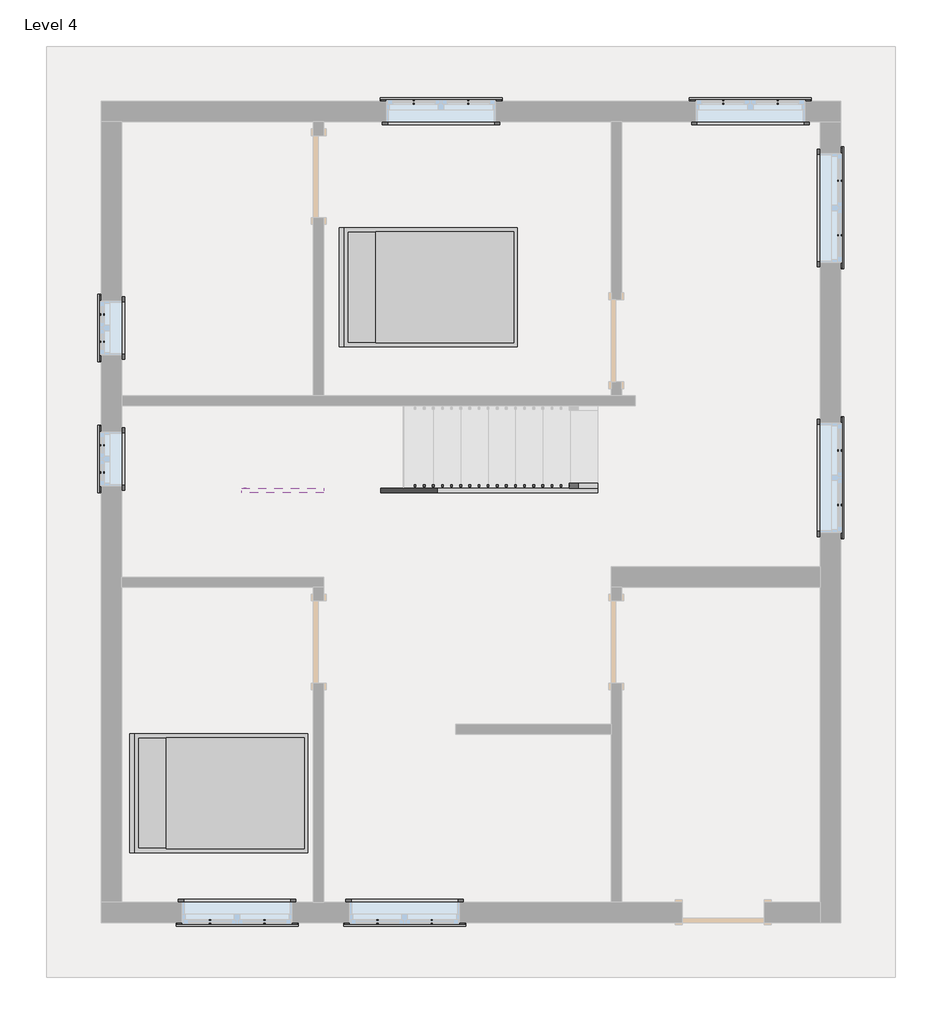
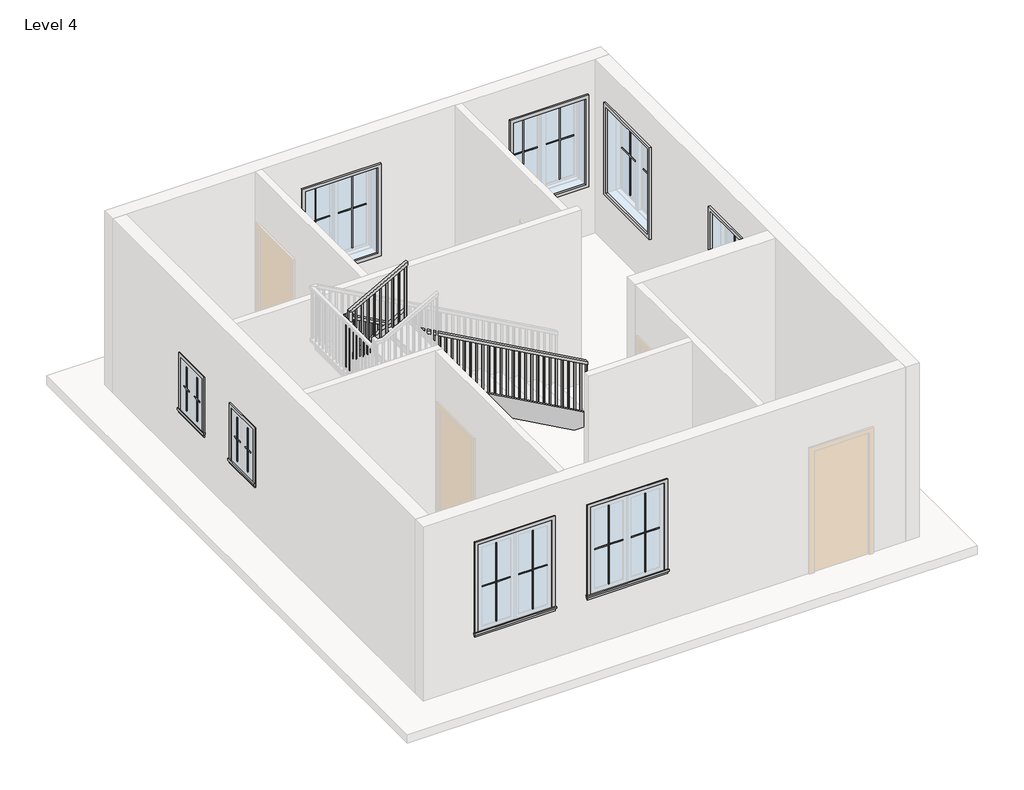
# One storey, part 2 of 2: 32 proxies, 3 members, 2 furniture elements, 1 railing.
"""IFC4 building model written with IfcOpenShell, lengths in millimetres."""

from ifc_helpers import new_model, si_unit, frame, origin, place, context, project, spatial, polyline, outline, extrude, faceted_brep, transform, mapped, element, save
from components import muntin_pattern_2x2_muntin_pattern_2x2_53152e2c, muntin_pattern_2x2_muntin_pattern_2x2_e8f3e573, muntin_pattern_2x2_muntin_pattern_2x2_6dad3731, muntin_pattern_2x2_muntin_pattern_2x2_a30a3345, trim_window_exterior_flat_with_sill_a665a915, trim_window_exterior_flat_with_sill_92b9b949, trim_window_interior_flat_picture_frame_d485c387, trim_window_interior_flat_picture_frame_3bb882cf, bed_17739_bed_17739_15c61121

model = new_model("IFC4")

# Units and contexts
model_context = context("Model", 3, world=origin())
ifc_project = project(units=[si_unit("LENGTHUNIT", "METRE", prefix="MILLI")], contexts=[model_context])

# Site, building, storey
site = spatial("IfcSite", under=ifc_project)
building = spatial("IfcBuilding", under=site)
storey = spatial("IfcBuildingStorey", under=building, Name="Level 4", Elevation=9144.0)

# Proxies
placement = place(None, origin())
muntin_pattern_2x2_muntin_pattern_2x2_shape = muntin_pattern_2x2_muntin_pattern_2x2_53152e2c(model_context)
element("IfcBuildingElementProxy", 1, Name="Muntin Pattern_2x2 : Muntin Pattern_2x2", ObjectType="Muntin Pattern_2x2 : Muntin Pattern_2x2", at=placement, inside=storey, context=model_context, shape_type="MappedRepresentation", body=[
    mapped(muntin_pattern_2x2_muntin_pattern_2x2_shape, transform((1279.525, 12101.9997886, 10128.25), x_axis=(0.0, 1.0, 0.0), y_axis=(-1.0, 0.0, 0.0), z_axis=(0.0, 0.0, 1.0))),
])
element("IfcBuildingElementProxy", 2, Name="Muntin Pattern_2x2 : Muntin Pattern_2x2", ObjectType="Muntin Pattern_2x2 : Muntin Pattern_2x2", at=placement, inside=storey, context=model_context, shape_type="MappedRepresentation", body=[
    mapped(muntin_pattern_2x2_muntin_pattern_2x2_shape, transform((1279.525, 10644.6747886, 10128.25), x_axis=(0.0, 1.0, 0.0), y_axis=(-1.0, 0.0, 0.0), z_axis=(0.0, 0.0, 1.0))),
])
muntin_pattern_2x2_muntin_pattern_2x2_2_shape = muntin_pattern_2x2_muntin_pattern_2x2_e8f3e573(model_context)
element("IfcBuildingElementProxy", 3, Name="Muntin Pattern_2x2 : Muntin Pattern_2x2", ObjectType="Muntin Pattern_2x2 : Muntin Pattern_2x2", at=placement, inside=storey, context=model_context, shape_type="MappedRepresentation", body=[
    mapped(muntin_pattern_2x2_muntin_pattern_2x2_2_shape, transform((1279.525, 12403.6247886, 10128.25), x_axis=(0.0, -1.0, 0.0), y_axis=(1.0, 0.0, 0.0), z_axis=(0.0, 0.0, 1.0))),
])
element("IfcBuildingElementProxy", 4, Name="Muntin Pattern_2x2 : Muntin Pattern_2x2", ObjectType="Muntin Pattern_2x2 : Muntin Pattern_2x2", at=placement, inside=storey, context=model_context, shape_type="MappedRepresentation", body=[
    mapped(muntin_pattern_2x2_muntin_pattern_2x2_2_shape, transform((1279.525, 10946.2997886, 10128.25), x_axis=(0.0, -1.0, 0.0), y_axis=(1.0, 0.0, 0.0), z_axis=(0.0, 0.0, 1.0))),
])
muntin_pattern_2x2_muntin_pattern_2x2_3_shape = muntin_pattern_2x2_muntin_pattern_2x2_6dad3731(model_context)
element("IfcBuildingElementProxy", 5, Name="Muntin Pattern_2x2 : Muntin Pattern_2x2", ObjectType="Muntin Pattern_2x2 : Muntin Pattern_2x2", at=placement, inside=storey, context=model_context, shape_type="MappedRepresentation", body=[
    mapped(muntin_pattern_2x2_muntin_pattern_2x2_3_shape, transform((9490.075, 13892.6997886, 10128.25), x_axis=(0.0, -1.0, 0.0), y_axis=(1.0, 0.0, 0.0), z_axis=(0.0, 0.0, 1.0))),
])
element("IfcBuildingElementProxy", 6, Name="Muntin Pattern_2x2 : Muntin Pattern_2x2", ObjectType="Muntin Pattern_2x2 : Muntin Pattern_2x2", at=placement, inside=storey, context=model_context, shape_type="MappedRepresentation", body=[
    mapped(muntin_pattern_2x2_muntin_pattern_2x2_3_shape, transform((8193.0875, 14767.4122886, 10128.25), x_axis=(1.0, 0.0, 0.0), y_axis=(0.0, 1.0, 0.0), z_axis=(0.0, 0.0, 1.0))),
])
element("IfcBuildingElementProxy", 7, Name="Muntin Pattern_2x2 : Muntin Pattern_2x2", ObjectType="Muntin Pattern_2x2 : Muntin Pattern_2x2", at=placement, inside=storey, context=model_context, shape_type="MappedRepresentation", body=[
    mapped(muntin_pattern_2x2_muntin_pattern_2x2_3_shape, transform((4749.8, 14767.4122886, 10128.25), x_axis=(1.0, 0.0, 0.0), y_axis=(0.0, 1.0, 0.0), z_axis=(0.0, 0.0, 1.0))),
])
element("IfcBuildingElementProxy", 8, Name="Muntin Pattern_2x2 : Muntin Pattern_2x2", ObjectType="Muntin Pattern_2x2 : Muntin Pattern_2x2", at=placement, inside=storey, context=model_context, shape_type="MappedRepresentation", body=[
    mapped(muntin_pattern_2x2_muntin_pattern_2x2_3_shape, transform((9490.075, 10889.1497886, 10128.25), x_axis=(0.0, -1.0, 0.0), y_axis=(1.0, 0.0, 0.0), z_axis=(0.0, 0.0, 1.0))),
])
element("IfcBuildingElementProxy", 9, Name="Muntin Pattern_2x2 : Muntin Pattern_2x2", ObjectType="Muntin Pattern_2x2 : Muntin Pattern_2x2", at=placement, inside=storey, context=model_context, shape_type="MappedRepresentation", body=[
    mapped(muntin_pattern_2x2_muntin_pattern_2x2_3_shape, transform((4950.6207347, 5642.4622886, 10128.25), x_axis=(-1.0, 0.0, 0.0), y_axis=(0.0, -1.0, 0.0), z_axis=(0.0, 0.0, 1.0))),
])
element("IfcBuildingElementProxy", 10, Name="Muntin Pattern_2x2 : Muntin Pattern_2x2", ObjectType="Muntin Pattern_2x2 : Muntin Pattern_2x2", at=placement, inside=storey, context=model_context, shape_type="MappedRepresentation", body=[
    mapped(muntin_pattern_2x2_muntin_pattern_2x2_3_shape, transform((3086.1019847, 5642.4622886, 10128.25), x_axis=(-1.0, 0.0, 0.0), y_axis=(0.0, -1.0, 0.0), z_axis=(0.0, 0.0, 1.0))),
])
muntin_pattern_2x2_muntin_pattern_2x2_4_shape = muntin_pattern_2x2_muntin_pattern_2x2_a30a3345(model_context)
element("IfcBuildingElementProxy", 11, Name="Muntin Pattern_2x2 : Muntin Pattern_2x2", ObjectType="Muntin Pattern_2x2 : Muntin Pattern_2x2", at=placement, inside=storey, context=model_context, shape_type="MappedRepresentation", body=[
    mapped(muntin_pattern_2x2_muntin_pattern_2x2_4_shape, transform((9490.075, 13286.2747886, 10128.25), x_axis=(0.0, 1.0, 0.0), y_axis=(-1.0, 0.0, 0.0), z_axis=(0.0, 0.0, 1.0))),
])
element("IfcBuildingElementProxy", 12, Name="Muntin Pattern_2x2 : Muntin Pattern_2x2", ObjectType="Muntin Pattern_2x2 : Muntin Pattern_2x2", at=placement, inside=storey, context=model_context, shape_type="MappedRepresentation", body=[
    mapped(muntin_pattern_2x2_muntin_pattern_2x2_4_shape, transform((8799.5125, 14767.4122886, 10128.25), x_axis=(-1.0, 0.0, 0.0), y_axis=(0.0, -1.0, 0.0), z_axis=(0.0, 0.0, 1.0))),
])
element("IfcBuildingElementProxy", 13, Name="Muntin Pattern_2x2 : Muntin Pattern_2x2", ObjectType="Muntin Pattern_2x2 : Muntin Pattern_2x2", at=placement, inside=storey, context=model_context, shape_type="MappedRepresentation", body=[
    mapped(muntin_pattern_2x2_muntin_pattern_2x2_4_shape, transform((5356.225, 14767.4122886, 10128.25), x_axis=(-1.0, 0.0, 0.0), y_axis=(0.0, -1.0, 0.0), z_axis=(0.0, 0.0, 1.0))),
])
element("IfcBuildingElementProxy", 14, Name="Muntin Pattern_2x2 : Muntin Pattern_2x2", ObjectType="Muntin Pattern_2x2 : Muntin Pattern_2x2", at=placement, inside=storey, context=model_context, shape_type="MappedRepresentation", body=[
    mapped(muntin_pattern_2x2_muntin_pattern_2x2_4_shape, transform((9490.075, 10282.7247886, 10128.25), x_axis=(0.0, 1.0, 0.0), y_axis=(-1.0, 0.0, 0.0), z_axis=(0.0, 0.0, 1.0))),
])
element("IfcBuildingElementProxy", 15, Name="Muntin Pattern_2x2 : Muntin Pattern_2x2", ObjectType="Muntin Pattern_2x2 : Muntin Pattern_2x2", at=placement, inside=storey, context=model_context, shape_type="MappedRepresentation", body=[
    mapped(muntin_pattern_2x2_muntin_pattern_2x2_4_shape, transform((4344.1957347, 5642.4622886, 10128.25), x_axis=(1.0, 0.0, 0.0), y_axis=(0.0, 1.0, 0.0), z_axis=(0.0, 0.0, 1.0))),
])
element("IfcBuildingElementProxy", 16, Name="Muntin Pattern_2x2 : Muntin Pattern_2x2", ObjectType="Muntin Pattern_2x2 : Muntin Pattern_2x2", at=placement, inside=storey, context=model_context, shape_type="MappedRepresentation", body=[
    mapped(muntin_pattern_2x2_muntin_pattern_2x2_4_shape, transform((2479.6769847, 5642.4622886, 10128.25), x_axis=(1.0, 0.0, 0.0), y_axis=(0.0, 1.0, 0.0), z_axis=(0.0, 0.0, 1.0))),
])
trim_window_exterior_flat_with_sill_shape = trim_window_exterior_flat_with_sill_a665a915(model_context)
element("IfcBuildingElementProxy", 17, Name="Trim-Window-Exterior-Flat : with Sill", ObjectType="Trim-Window-Exterior-Flat : with Sill", at=placement, inside=storey, context=model_context, shape_type="MappedRepresentation", body=[
    mapped(trim_window_exterior_flat_with_sill_shape, transform((1270.0, 12252.8122886, 10972.8), x_axis=(0.0, -1.0, 0.0), y_axis=(0.0, 0.0, 1.0), z_axis=(-1.0, 0.0, 0.0))),
])
element("IfcBuildingElementProxy", 18, Name="Trim-Window-Exterior-Flat : with Sill", ObjectType="Trim-Window-Exterior-Flat : with Sill", at=placement, inside=storey, context=model_context, shape_type="MappedRepresentation", body=[
    mapped(trim_window_exterior_flat_with_sill_shape, transform((1270.0, 10795.4872886, 10972.8), x_axis=(0.0, -1.0, 0.0), y_axis=(0.0, 0.0, 1.0), z_axis=(-1.0, 0.0, 0.0))),
])
trim_window_exterior_flat_with_sill_2_shape = trim_window_exterior_flat_with_sill_92b9b949(model_context)
element("IfcBuildingElementProxy", 19, Name="Trim-Window-Exterior-Flat : with Sill", ObjectType="Trim-Window-Exterior-Flat : with Sill", at=placement, inside=storey, context=model_context, shape_type="MappedRepresentation", body=[
    mapped(trim_window_exterior_flat_with_sill_2_shape, transform((9499.6, 13589.4872886, 11582.4), x_axis=(0.0, 1.0, 0.0), y_axis=(0.0, 0.0, 1.0), z_axis=(1.0, 0.0, 0.0))),
])
element("IfcBuildingElementProxy", 20, Name="Trim-Window-Exterior-Flat : with Sill", ObjectType="Trim-Window-Exterior-Flat : with Sill", at=placement, inside=storey, context=model_context, shape_type="MappedRepresentation", body=[
    mapped(trim_window_exterior_flat_with_sill_2_shape, transform((8496.3, 14776.9372886, 11582.4), x_axis=(-1.0, 0.0, 0.0), y_axis=(0.0, 0.0, 1.0), z_axis=(0.0, 1.0, 0.0))),
])
element("IfcBuildingElementProxy", 21, Name="Trim-Window-Exterior-Flat : with Sill", ObjectType="Trim-Window-Exterior-Flat : with Sill", at=placement, inside=storey, context=model_context, shape_type="MappedRepresentation", body=[
    mapped(trim_window_exterior_flat_with_sill_2_shape, transform((5053.0125, 14776.9372886, 11582.4), x_axis=(-1.0, 0.0, 0.0), y_axis=(0.0, 0.0, 1.0), z_axis=(0.0, 1.0, 0.0))),
])
element("IfcBuildingElementProxy", 22, Name="Trim-Window-Exterior-Flat : with Sill", ObjectType="Trim-Window-Exterior-Flat : with Sill", at=placement, inside=storey, context=model_context, shape_type="MappedRepresentation", body=[
    mapped(trim_window_exterior_flat_with_sill_2_shape, transform((9499.6, 10585.9372886, 11582.4), x_axis=(0.0, 1.0, 0.0), y_axis=(0.0, 0.0, 1.0), z_axis=(1.0, 0.0, 0.0))),
])
element("IfcBuildingElementProxy", 23, Name="Trim-Window-Exterior-Flat : with Sill", ObjectType="Trim-Window-Exterior-Flat : with Sill", at=placement, inside=storey, context=model_context, shape_type="MappedRepresentation", body=[
    mapped(trim_window_exterior_flat_with_sill_2_shape, transform((4647.4082347, 5632.9372886, 11582.4), x_axis=(1.0, 0.0, 0.0), y_axis=(0.0, 0.0, 1.0), z_axis=(0.0, -1.0, 0.0))),
])
element("IfcBuildingElementProxy", 24, Name="Trim-Window-Exterior-Flat : with Sill", ObjectType="Trim-Window-Exterior-Flat : with Sill", at=placement, inside=storey, context=model_context, shape_type="MappedRepresentation", body=[
    mapped(trim_window_exterior_flat_with_sill_2_shape, transform((2782.8894847, 5632.9372886, 11582.4), x_axis=(1.0, 0.0, 0.0), y_axis=(0.0, 0.0, 1.0), z_axis=(0.0, -1.0, 0.0))),
])
trim_window_interior_flat_picture_frame_shape = trim_window_interior_flat_picture_frame_d485c387(model_context)
element("IfcBuildingElementProxy", 25, Name="Trim-Window-Interior-Flat : Picture Frame", ObjectType="Trim-Window-Interior-Flat : Picture Frame", at=placement, inside=storey, context=model_context, shape_type="MappedRepresentation", body=[
    mapped(trim_window_interior_flat_picture_frame_shape, transform((1498.6, 12252.8122886, 10972.8), x_axis=(0.0, 1.0, 0.0), y_axis=(0.0, 0.0, 1.0), z_axis=(1.0, 0.0, 0.0))),
])
element("IfcBuildingElementProxy", 26, Name="Trim-Window-Interior-Flat : Picture Frame", ObjectType="Trim-Window-Interior-Flat : Picture Frame", at=placement, inside=storey, context=model_context, shape_type="MappedRepresentation", body=[
    mapped(trim_window_interior_flat_picture_frame_shape, transform((1498.6, 10795.4872886, 10972.8), x_axis=(0.0, 1.0, 0.0), y_axis=(0.0, 0.0, 1.0), z_axis=(1.0, 0.0, 0.0))),
])
trim_window_interior_flat_picture_frame_2_shape = trim_window_interior_flat_picture_frame_3bb882cf(model_context)
element("IfcBuildingElementProxy", 27, Name="Trim-Window-Interior-Flat : Picture Frame", ObjectType="Trim-Window-Interior-Flat : Picture Frame", at=placement, inside=storey, context=model_context, shape_type="MappedRepresentation", body=[
    mapped(trim_window_interior_flat_picture_frame_2_shape, transform((9271.0, 13589.4872886, 11582.4), x_axis=(0.0, -1.0, 0.0), y_axis=(0.0, 0.0, 1.0), z_axis=(-1.0, 0.0, 0.0))),
])
element("IfcBuildingElementProxy", 28, Name="Trim-Window-Interior-Flat : Picture Frame", ObjectType="Trim-Window-Interior-Flat : Picture Frame", at=placement, inside=storey, context=model_context, shape_type="MappedRepresentation", body=[
    mapped(trim_window_interior_flat_picture_frame_2_shape, transform((8496.3, 14548.3372886, 11582.4), x_axis=(1.0, 0.0, 0.0), y_axis=(0.0, 0.0, 1.0), z_axis=(0.0, -1.0, 0.0))),
])
element("IfcBuildingElementProxy", 29, Name="Trim-Window-Interior-Flat : Picture Frame", ObjectType="Trim-Window-Interior-Flat : Picture Frame", at=placement, inside=storey, context=model_context, shape_type="MappedRepresentation", body=[
    mapped(trim_window_interior_flat_picture_frame_2_shape, transform((5053.0125, 14548.3372886, 11582.4), x_axis=(1.0, 0.0, 0.0), y_axis=(0.0, 0.0, 1.0), z_axis=(0.0, -1.0, 0.0))),
])
element("IfcBuildingElementProxy", 30, Name="Trim-Window-Interior-Flat : Picture Frame", ObjectType="Trim-Window-Interior-Flat : Picture Frame", at=placement, inside=storey, context=model_context, shape_type="MappedRepresentation", body=[
    mapped(trim_window_interior_flat_picture_frame_2_shape, transform((9271.0, 10585.9372886, 11582.4), x_axis=(0.0, -1.0, 0.0), y_axis=(0.0, 0.0, 1.0), z_axis=(-1.0, 0.0, 0.0))),
])
element("IfcBuildingElementProxy", 31, Name="Trim-Window-Interior-Flat : Picture Frame", ObjectType="Trim-Window-Interior-Flat : Picture Frame", at=placement, inside=storey, context=model_context, shape_type="MappedRepresentation", body=[
    mapped(trim_window_interior_flat_picture_frame_2_shape, transform((4647.4082347, 5861.5372886, 11582.4), x_axis=(-1.0, 0.0, 0.0), y_axis=(0.0, 0.0, 1.0), z_axis=(0.0, 1.0, 0.0))),
])
element("IfcBuildingElementProxy", 32, Name="Trim-Window-Interior-Flat : Picture Frame", ObjectType="Trim-Window-Interior-Flat : Picture Frame", at=placement, inside=storey, context=model_context, shape_type="MappedRepresentation", body=[
    mapped(trim_window_interior_flat_picture_frame_2_shape, transform((2782.8894847, 5861.5372886, 11582.4), x_axis=(-1.0, 0.0, 0.0), y_axis=(0.0, 0.0, 1.0), z_axis=(0.0, 1.0, 0.0))),
])

# Furniture
bed_17739_bed_17739_shape = bed_17739_bed_17739_15c61121(model_context)
element("IfcFurniture", 33, ObjectType="Bed_17739 : Bed_17739", at=placement, inside=storey, context=model_context, shape_type="MappedRepresentation", body=[
    mapped(bed_17739_bed_17739_shape, transform((4933.95, 12706.8372886, 9144.0), x_axis=(0.0, 1.0, 0.0), y_axis=(-1.0, 0.0, 0.0), z_axis=(0.0, 0.0, 1.0))),
])
element("IfcFurniture", 34, ObjectType="Bed_17739 : Bed_17739", at=placement, inside=storey, context=model_context, shape_type="MappedRepresentation", body=[
    mapped(bed_17739_bed_17739_shape, transform((2603.5, 7074.3872886, 9144.0), x_axis=(0.0, 1.0, 0.0), y_axis=(-1.0, 0.0, 0.0), z_axis=(0.0, 0.0, 1.0))),
])

# Members
element("IfcMember", 35, ObjectType="Stringer - 2\" Width", at=placement, inside=storey, context=model_context, shape_type="SweptSolid", body=[
    extrude(outline(polyline([(9144.0, 6794.5), (9351.5983948, 6794.5), (11524.7095059, 2882.9), (11176.0308318, 2882.9), (9144.0, 6540.5554972), (9144.0, 6794.5)])), frame((0.0, 10420.8372886, 0.0), z_axis=(0.0, 1.0, 0.0), x_axis=(0.0, 0.0, 1.0)), (0.0, 0.0, 1.0), 50.8),
])
element("IfcMember", 36, ObjectType="Stringer - 2\" Width", at=placement, inside=storey, context=model_context, shape_type="SweptSolid", body=[
    extrude(outline(polyline([(2832.1, 10471.6372886), (2882.9, 10471.6372886), (2882.9, 10469.0972886), (2832.1, 10469.0972886), (2832.1, 10471.6372886)])), frame((0.0, 0.0, 11286.0666667), z_axis=(0.0, 0.0, 1.0), x_axis=(1.0, 0.0, 0.0)), (0.0, 0.0, 1.0), 304.8),
])
element("IfcMember", 37, ObjectType="Stringer - 2\" Width", at=placement, inside=storey, context=model_context, shape_type="SweptSolid", body=[
    extrude(outline(polyline([(11722.2650614, 2832.1), (11373.5863873, 2832.1), (11881.5874899, 3746.5019847), (12230.266164, 3746.5019847), (11722.2650614, 2832.1)])), frame((0.0, 10418.2972886, 0.0), z_axis=(0.0, 1.0, 0.0), x_axis=(0.0, 0.0, 1.0)), (0.0, 0.0, 1.0), 50.8),
])

# Railing
element("IfcRailing", 38, ObjectType="Handrail - Rectangular", at=placement, inside=storey, context=model_context, shape_type="SolidModel", body=[
    faceted_brep([(6794.5, 10471.6372886, 10227.7333333), (6794.5, 10471.6372886, 10169.620221), (6794.5, 10522.4372886, 10169.620221), (6794.5, 10522.4372886, 10227.7333333), (2908.3, 10471.6372886, 12386.7333333), (2857.5, 10471.6372886, 12356.8424432), (2857.5, 10522.4372886, 12356.8424432), (2908.3, 10522.4372886, 12386.7333333), (2908.3, 10471.6372886, 12429.0666667), (2857.5, 10471.6372886, 12378.2666667), (2857.5, 10522.4372886, 12378.2666667), (2908.3, 10522.4372886, 12429.0666667), (2832.1, 10471.6372886, 12429.0666667), (2832.1, 10471.6372886, 12378.2666667), (2781.3, 10522.4372886, 12378.2666667), (2781.3, 10522.4372886, 12429.0666667), (2832.1, 10395.4372886, 12429.0666667), (2832.1, 10395.4372886, 12378.2666667), (2781.3, 10395.4372886, 12378.2666667), (2781.3, 10395.4372886, 12429.0666667), (2832.1, 10392.8972886, 12429.0666667), (2781.3, 10392.8972886, 12429.0666667), (2781.3, 10392.8972886, 12378.2666667), (2832.1, 10392.8972886, 12378.2666667)], [[[0, 1, 2, 3]], [[1, 0, 4, 5]], [[2, 1, 5, 6]], [[3, 2, 6, 7]], [[0, 3, 7, 4]], [[5, 4, 8, 9]], [[6, 5, 9, 10]], [[7, 6, 10, 11]], [[4, 7, 11, 8]], [[9, 8, 12, 13]], [[10, 9, 13, 14]], [[11, 10, 14, 15]], [[8, 11, 15, 12]], [[13, 12, 16, 17]], [[14, 13, 17, 18]], [[15, 14, 18, 19]], [[12, 15, 19, 16]], [[20, 21, 22, 23]], [[17, 16, 20, 23]], [[18, 17, 23, 22]], [[19, 18, 22, 21]], [[16, 19, 21, 20]]]),
    faceted_brep([(2832.1, 10418.2972886, 12429.0666667), (2832.1, 10367.4972886, 12378.2666667), (2781.3, 10367.4972886, 12378.2666667), (2781.3, 10418.2972886, 12429.0666667), (2832.1, 10418.2972886, 12540.2869174), (2781.3, 10418.2972886, 12570.177839), (2781.3, 10367.4972886, 12570.177839), (2832.1, 10367.4972886, 12540.2869174)], [[[0, 1, 2, 3]], [[4, 5, 6, 7]], [[1, 0, 4, 7]], [[2, 1, 7, 6]], [[3, 2, 6, 5]], [[0, 3, 5, 4]]]),
    faceted_brep([(2781.3, 10418.2972886, 12570.177839), (2832.1, 10418.2972886, 12540.2869174), (2832.1, 10367.4972886, 12540.2869174), (2781.3, 10367.4972886, 12570.177839), (3746.5019847, 10418.2972886, 13106.4), (3746.5019847, 10367.4972886, 13106.4), (3746.5019847, 10367.4972886, 13048.2869174), (3746.5019847, 10418.2972886, 13048.2869174)], [[[0, 1, 2, 3]], [[4, 5, 6, 7]], [[1, 0, 4, 7]], [[2, 1, 7, 6]], [[3, 2, 6, 5]], [[0, 3, 5, 4]]]),
    extrude(outline(polyline([(13028.8838142, 3711.575), (12022.6666667, 3711.575), (12022.6666667, 3730.625), (13039.4671246, 3730.625), (13028.8838142, 3711.575)])), frame((0.0, 10383.3722886, 0.0), z_axis=(0.0, 1.0, 0.0), x_axis=(0.0, 0.0, 1.0)), (0.0, 0.0, 1.0), 19.05),
    extrude(outline(polyline([(12972.4394923, 3609.975), (12022.6666667, 3609.975), (12022.6666667, 3629.025), (12983.0228026, 3629.025), (12972.4394923, 3609.975)])), frame((0.0, 10383.3722886, 0.0), z_axis=(0.0, 1.0, 0.0), x_axis=(0.0, 0.0, 1.0)), (0.0, 0.0, 1.0), 19.05),
    extrude(outline(polyline([(12915.9951703, 3508.375), (12022.6666667, 3508.375), (12022.6666667, 3527.425), (12926.5784807, 3527.425), (12915.9951703, 3508.375)])), frame((0.0, 10383.3722886, 0.0), z_axis=(0.0, 1.0, 0.0), x_axis=(0.0, 0.0, 1.0)), (0.0, 0.0, 1.0), 19.05),
    extrude(outline(polyline([(12859.5504809, 3406.775), (11853.3333333, 3406.775), (11853.3333333, 3425.825), (12870.1337912, 3425.825), (12859.5504809, 3406.775)])), frame((0.0, 10383.3722886, 0.0), z_axis=(0.0, 1.0, 0.0), x_axis=(0.0, 0.0, 1.0)), (0.0, 0.0, 1.0), 19.05),
    extrude(outline(polyline([(12803.1061589, 3305.175), (11853.3333333, 3305.175), (11853.3333333, 3324.225), (12813.6894693, 3324.225), (12803.1061589, 3305.175)])), frame((0.0, 10383.3722886, 0.0), z_axis=(0.0, 1.0, 0.0), x_axis=(0.0, 0.0, 1.0)), (0.0, 0.0, 1.0), 19.05),
    extrude(outline(polyline([(12746.661837, 3203.575), (11853.3333333, 3203.575), (11853.3333333, 3222.625), (12757.2451474, 3222.625), (12746.661837, 3203.575)])), frame((0.0, 10383.3722886, 0.0), z_axis=(0.0, 1.0, 0.0), x_axis=(0.0, 0.0, 1.0)), (0.0, 0.0, 1.0), 19.05),
    extrude(outline(polyline([(12690.2171475, 3101.975), (11684.0, 3101.975), (11684.0, 3121.025), (12700.8004579, 3121.025), (12690.2171475, 3101.975)])), frame((0.0, 10383.3722886, 0.0), z_axis=(0.0, 1.0, 0.0), x_axis=(0.0, 0.0, 1.0)), (0.0, 0.0, 1.0), 19.05),
    extrude(outline(polyline([(12633.7728256, 3000.375), (11684.0, 3000.375), (11684.0, 3019.425), (12644.356136, 3019.425), (12633.7728256, 3000.375)])), frame((0.0, 10383.3722886, 0.0), z_axis=(0.0, 1.0, 0.0), x_axis=(0.0, 0.0, 1.0)), (0.0, 0.0, 1.0), 19.05),
    extrude(outline(polyline([(12577.3285037, 2898.775), (11684.0, 2898.775), (11684.0, 2917.825), (12587.911814, 2917.825), (12577.3285037, 2898.775)])), frame((0.0, 10383.3722886, 0.0), z_axis=(0.0, 1.0, 0.0), x_axis=(0.0, 0.0, 1.0)), (0.0, 0.0, 1.0), 19.05),
    extrude(outline(polyline([(2816.225, 10404.9622886), (2816.225, 10385.9122886), (2797.175, 10385.9122886), (2797.175, 10404.9622886), (2816.225, 10404.9622886)])), frame((0.0, 0.0, 11514.6666667), z_axis=(0.0, 0.0, 1.0), x_axis=(1.0, 0.0, 0.0)), (0.0, 0.0, 1.0), 863.6),
    extrude(outline(polyline([(2841.625, 10487.5122886), (2822.575, 10487.5122886), (2822.575, 10506.5622886), (2841.625, 10506.5622886), (2841.625, 10487.5122886)])), frame((0.0, 0.0, 11514.6666667), z_axis=(0.0, 0.0, 1.0), x_axis=(1.0, 0.0, 0.0)), (0.0, 0.0, 1.0), 863.6),
    extrude(outline(polyline([(12319.8007765, 2924.175), (11345.3333333, 2924.175), (11345.3333333, 2943.225), (12309.2174432, 2943.225), (12319.8007765, 2924.175)])), frame((0.0, 10487.5122886, 0.0), z_axis=(0.0, 1.0, 0.0), x_axis=(0.0, 0.0, 1.0)), (0.0, 0.0, 1.0), 19.05),
    extrude(outline(polyline([(12263.3563321, 3025.775), (11345.3333333, 3025.775), (11345.3333333, 3044.825), (12252.7729988, 3044.825), (12263.3563321, 3025.775)])), frame((0.0, 10487.5122886, 0.0), z_axis=(0.0, 1.0, 0.0), x_axis=(0.0, 0.0, 1.0)), (0.0, 0.0, 1.0), 19.05),
    extrude(outline(polyline([(12206.9118876, 3127.375), (11345.3333333, 3127.375), (11345.3333333, 3146.425), (12196.3285543, 3146.425), (12206.9118876, 3127.375)])), frame((0.0, 10487.5122886, 0.0), z_axis=(0.0, 1.0, 0.0), x_axis=(0.0, 0.0, 1.0)), (0.0, 0.0, 1.0), 19.05),
    extrude(outline(polyline([(12150.4674432, 3228.975), (11176.0, 3228.975), (11176.0, 3248.025), (12139.8841099, 3248.025), (12150.4674432, 3228.975)])), frame((0.0, 10487.5122886, 0.0), z_axis=(0.0, 1.0, 0.0), x_axis=(0.0, 0.0, 1.0)), (0.0, 0.0, 1.0), 19.05),
    extrude(outline(polyline([(12094.0229988, 3330.575), (11176.0, 3330.575), (11176.0, 3349.625), (12083.4396654, 3349.625), (12094.0229988, 3330.575)])), frame((0.0, 10487.5122886, 0.0), z_axis=(0.0, 1.0, 0.0), x_axis=(0.0, 0.0, 1.0)), (0.0, 0.0, 1.0), 19.05),
    extrude(outline(polyline([(12037.5785543, 3432.175), (11176.0, 3432.175), (11176.0, 3451.225), (12026.995221, 3451.225), (12037.5785543, 3432.175)])), frame((0.0, 10487.5122886, 0.0), z_axis=(0.0, 1.0, 0.0), x_axis=(0.0, 0.0, 1.0)), (0.0, 0.0, 1.0), 19.05),
    extrude(outline(polyline([(11981.1341099, 3533.775), (11006.6666667, 3533.775), (11006.6666667, 3552.825), (11970.5507765, 3552.825), (11981.1341099, 3533.775)])), frame((0.0, 10487.5122886, 0.0), z_axis=(0.0, 1.0, 0.0), x_axis=(0.0, 0.0, 1.0)), (0.0, 0.0, 1.0), 19.05),
    extrude(outline(polyline([(11924.6896654, 3635.375), (11006.6666667, 3635.375), (11006.6666667, 3654.425), (11914.1063321, 3654.425), (11924.6896654, 3635.375)])), frame((0.0, 10487.5122886, 0.0), z_axis=(0.0, 1.0, 0.0), x_axis=(0.0, 0.0, 1.0)), (0.0, 0.0, 1.0), 19.05),
    extrude(outline(polyline([(11868.245221, 3736.975), (11006.6666667, 3736.975), (11006.6666667, 3756.025), (11857.6618876, 3756.025), (11868.245221, 3736.975)])), frame((0.0, 10487.5122886, 0.0), z_axis=(0.0, 1.0, 0.0), x_axis=(0.0, 0.0, 1.0)), (0.0, 0.0, 1.0), 19.05),
    extrude(outline(polyline([(11811.8007765, 3838.575), (10837.3333333, 3838.575), (10837.3333333, 3857.625), (11801.2174432, 3857.625), (11811.8007765, 3838.575)])), frame((0.0, 10487.5122886, 0.0), z_axis=(0.0, 1.0, 0.0), x_axis=(0.0, 0.0, 1.0)), (0.0, 0.0, 1.0), 19.05),
    extrude(outline(polyline([(11755.3563321, 3940.175), (10837.3333333, 3940.175), (10837.3333333, 3959.225), (11744.7729988, 3959.225), (11755.3563321, 3940.175)])), frame((0.0, 10487.5122886, 0.0), z_axis=(0.0, 1.0, 0.0), x_axis=(0.0, 0.0, 1.0)), (0.0, 0.0, 1.0), 19.05),
    extrude(outline(polyline([(11698.9118876, 4041.775), (10837.3333333, 4041.775), (10837.3333333, 4060.825), (11688.3285543, 4060.825), (11698.9118876, 4041.775)])), frame((0.0, 10487.5122886, 0.0), z_axis=(0.0, 1.0, 0.0), x_axis=(0.0, 0.0, 1.0)), (0.0, 0.0, 1.0), 19.05),
    extrude(outline(polyline([(11642.4674432, 4143.375), (10668.0, 4143.375), (10668.0, 4162.425), (11631.8841099, 4162.425), (11642.4674432, 4143.375)])), frame((0.0, 10487.5122886, 0.0), z_axis=(0.0, 1.0, 0.0), x_axis=(0.0, 0.0, 1.0)), (0.0, 0.0, 1.0), 19.05),
    extrude(outline(polyline([(11586.0229988, 4244.975), (10668.0, 4244.975), (10668.0, 4264.025), (11575.4396654, 4264.025), (11586.0229988, 4244.975)])), frame((0.0, 10487.5122886, 0.0), z_axis=(0.0, 1.0, 0.0), x_axis=(0.0, 0.0, 1.0)), (0.0, 0.0, 1.0), 19.05),
    extrude(outline(polyline([(11529.5785543, 4346.575), (10668.0, 4346.575), (10668.0, 4365.625), (11518.995221, 4365.625), (11529.5785543, 4346.575)])), frame((0.0, 10487.5122886, 0.0), z_axis=(0.0, 1.0, 0.0), x_axis=(0.0, 0.0, 1.0)), (0.0, 0.0, 1.0), 19.05),
    extrude(outline(polyline([(11473.1341099, 4448.175), (10498.6666667, 4448.175), (10498.6666667, 4467.225), (11462.5507765, 4467.225), (11473.1341099, 4448.175)])), frame((0.0, 10487.5122886, 0.0), z_axis=(0.0, 1.0, 0.0), x_axis=(0.0, 0.0, 1.0)), (0.0, 0.0, 1.0), 19.05),
    extrude(outline(polyline([(11416.6896654, 4549.775), (10498.6666667, 4549.775), (10498.6666667, 4568.825), (11406.1063321, 4568.825), (11416.6896654, 4549.775)])), frame((0.0, 10487.5122886, 0.0), z_axis=(0.0, 1.0, 0.0), x_axis=(0.0, 0.0, 1.0)), (0.0, 0.0, 1.0), 19.05),
    extrude(outline(polyline([(11360.245221, 4651.375), (10498.6666667, 4651.375), (10498.6666667, 4670.425), (11349.6618876, 4670.425), (11360.245221, 4651.375)])), frame((0.0, 10487.5122886, 0.0), z_axis=(0.0, 1.0, 0.0), x_axis=(0.0, 0.0, 1.0)), (0.0, 0.0, 1.0), 19.05),
    extrude(outline(polyline([(11303.8007765, 4752.975), (10329.3333333, 4752.975), (10329.3333333, 4772.025), (11293.2174432, 4772.025), (11303.8007765, 4752.975)])), frame((0.0, 10487.5122886, 0.0), z_axis=(0.0, 1.0, 0.0), x_axis=(0.0, 0.0, 1.0)), (0.0, 0.0, 1.0), 19.05),
    extrude(outline(polyline([(11247.3563321, 4854.575), (10329.3333333, 4854.575), (10329.3333333, 4873.625), (11236.7729988, 4873.625), (11247.3563321, 4854.575)])), frame((0.0, 10487.5122886, 0.0), z_axis=(0.0, 1.0, 0.0), x_axis=(0.0, 0.0, 1.0)), (0.0, 0.0, 1.0), 19.05),
    extrude(outline(polyline([(11190.9118876, 4956.175), (10329.3333333, 4956.175), (10329.3333333, 4975.225), (11180.3285543, 4975.225), (11190.9118876, 4956.175)])), frame((0.0, 10487.5122886, 0.0), z_axis=(0.0, 1.0, 0.0), x_axis=(0.0, 0.0, 1.0)), (0.0, 0.0, 1.0), 19.05),
    extrude(outline(polyline([(11134.4674432, 5057.775), (10160.0, 5057.775), (10160.0, 5076.825), (11123.8841099, 5076.825), (11134.4674432, 5057.775)])), frame((0.0, 10487.5122886, 0.0), z_axis=(0.0, 1.0, 0.0), x_axis=(0.0, 0.0, 1.0)), (0.0, 0.0, 1.0), 19.05),
    extrude(outline(polyline([(11078.0229988, 5159.375), (10160.0, 5159.375), (10160.0, 5178.425), (11067.4396654, 5178.425), (11078.0229988, 5159.375)])), frame((0.0, 10487.5122886, 0.0), z_axis=(0.0, 1.0, 0.0), x_axis=(0.0, 0.0, 1.0)), (0.0, 0.0, 1.0), 19.05),
    extrude(outline(polyline([(11021.5785543, 5260.975), (10160.0, 5260.975), (10160.0, 5280.025), (11010.995221, 5280.025), (11021.5785543, 5260.975)])), frame((0.0, 10487.5122886, 0.0), z_axis=(0.0, 1.0, 0.0), x_axis=(0.0, 0.0, 1.0)), (0.0, 0.0, 1.0), 19.05),
    extrude(outline(polyline([(10965.1341099, 5362.575), (9990.6666667, 5362.575), (9990.6666667, 5381.625), (10954.5507765, 5381.625), (10965.1341099, 5362.575)])), frame((0.0, 10487.5122886, 0.0), z_axis=(0.0, 1.0, 0.0), x_axis=(0.0, 0.0, 1.0)), (0.0, 0.0, 1.0), 19.05),
    extrude(outline(polyline([(10908.6896654, 5464.175), (9990.6666667, 5464.175), (9990.6666667, 5483.225), (10898.1063321, 5483.225), (10908.6896654, 5464.175)])), frame((0.0, 10487.5122886, 0.0), z_axis=(0.0, 1.0, 0.0), x_axis=(0.0, 0.0, 1.0)), (0.0, 0.0, 1.0), 19.05),
    extrude(outline(polyline([(10852.245221, 5565.775), (9990.6666667, 5565.775), (9990.6666667, 5584.825), (10841.6618876, 5584.825), (10852.245221, 5565.775)])), frame((0.0, 10487.5122886, 0.0), z_axis=(0.0, 1.0, 0.0), x_axis=(0.0, 0.0, 1.0)), (0.0, 0.0, 1.0), 19.05),
    extrude(outline(polyline([(10795.8007765, 5667.375), (9821.3333333, 5667.375), (9821.3333333, 5686.425), (10785.2174432, 5686.425), (10795.8007765, 5667.375)])), frame((0.0, 10487.5122886, 0.0), z_axis=(0.0, 1.0, 0.0), x_axis=(0.0, 0.0, 1.0)), (0.0, 0.0, 1.0), 19.05),
    extrude(outline(polyline([(10739.3563321, 5768.975), (9821.3333333, 5768.975), (9821.3333333, 5788.025), (10728.7729988, 5788.025), (10739.3563321, 5768.975)])), frame((0.0, 10487.5122886, 0.0), z_axis=(0.0, 1.0, 0.0), x_axis=(0.0, 0.0, 1.0)), (0.0, 0.0, 1.0), 19.05),
    extrude(outline(polyline([(10682.9118876, 5870.575), (9821.3333333, 5870.575), (9821.3333333, 5889.625), (10672.3285543, 5889.625), (10682.9118876, 5870.575)])), frame((0.0, 10487.5122886, 0.0), z_axis=(0.0, 1.0, 0.0), x_axis=(0.0, 0.0, 1.0)), (0.0, 0.0, 1.0), 19.05),
    extrude(outline(polyline([(10626.4674432, 5972.175), (9652.0, 5972.175), (9652.0, 5991.225), (10615.8841099, 5991.225), (10626.4674432, 5972.175)])), frame((0.0, 10487.5122886, 0.0), z_axis=(0.0, 1.0, 0.0), x_axis=(0.0, 0.0, 1.0)), (0.0, 0.0, 1.0), 19.05),
    extrude(outline(polyline([(10570.0229988, 6073.775), (9652.0, 6073.775), (9652.0, 6092.825), (10559.4396654, 6092.825), (10570.0229988, 6073.775)])), frame((0.0, 10487.5122886, 0.0), z_axis=(0.0, 1.0, 0.0), x_axis=(0.0, 0.0, 1.0)), (0.0, 0.0, 1.0), 19.05),
    extrude(outline(polyline([(10513.5785543, 6175.375), (9652.0, 6175.375), (9652.0, 6194.425), (10502.995221, 6194.425), (10513.5785543, 6175.375)])), frame((0.0, 10487.5122886, 0.0), z_axis=(0.0, 1.0, 0.0), x_axis=(0.0, 0.0, 1.0)), (0.0, 0.0, 1.0), 19.05),
    extrude(outline(polyline([(10457.1341099, 6276.975), (9482.6666667, 6276.975), (9482.6666667, 6296.025), (10446.5507765, 6296.025), (10457.1341099, 6276.975)])), frame((0.0, 10487.5122886, 0.0), z_axis=(0.0, 1.0, 0.0), x_axis=(0.0, 0.0, 1.0)), (0.0, 0.0, 1.0), 19.05),
    extrude(outline(polyline([(10400.6896654, 6378.575), (9482.6666667, 6378.575), (9482.6666667, 6397.625), (10390.1063321, 6397.625), (10400.6896654, 6378.575)])), frame((0.0, 10487.5122886, 0.0), z_axis=(0.0, 1.0, 0.0), x_axis=(0.0, 0.0, 1.0)), (0.0, 0.0, 1.0), 19.05),
    extrude(outline(polyline([(10344.245221, 6480.175), (9482.6666667, 6480.175), (9482.6666667, 6499.225), (10333.6618876, 6499.225), (10344.245221, 6480.175)])), frame((0.0, 10487.5122886, 0.0), z_axis=(0.0, 1.0, 0.0), x_axis=(0.0, 0.0, 1.0)), (0.0, 0.0, 1.0), 19.05),
    extrude(outline(polyline([(10287.8007765, 6581.775), (9313.3333333, 6581.775), (9313.3333333, 6600.825), (10277.2174432, 6600.825), (10287.8007765, 6581.775)])), frame((0.0, 10487.5122886, 0.0), z_axis=(0.0, 1.0, 0.0), x_axis=(0.0, 0.0, 1.0)), (0.0, 0.0, 1.0), 19.05),
    extrude(outline(polyline([(10231.3563321, 6683.375), (9313.3333333, 6683.375), (9313.3333333, 6702.425), (10220.7729988, 6702.425), (10231.3563321, 6683.375)])), frame((0.0, 10487.5122886, 0.0), z_axis=(0.0, 1.0, 0.0), x_axis=(0.0, 0.0, 1.0)), (0.0, 0.0, 1.0), 19.05),
    extrude(outline(polyline([(2816.225, 10402.4222886), (2816.225, 10383.3722886), (2797.175, 10383.3722886), (2797.175, 10402.4222886), (2816.225, 10402.4222886)])), frame((0.0, 0.0, 11514.6666667), z_axis=(0.0, 0.0, 1.0), x_axis=(1.0, 0.0, 0.0)), (0.0, 0.0, 1.0), 863.6),
    extrude(outline(polyline([(2816.225, 10487.5122886), (2797.175, 10487.5122886), (2797.175, 10506.5622886), (2816.225, 10506.5622886), (2816.225, 10487.5122886)])), frame((0.0, 0.0, 11514.6666667), z_axis=(0.0, 0.0, 1.0), x_axis=(1.0, 0.0, 0.0)), (0.0, 0.0, 1.0), 863.6),
    extrude(outline(polyline([(13037.703607, 3727.4519847), (12022.6666667, 3727.4519847), (12022.6666667, 3746.5019847), (13048.2869174, 3746.5019847), (13037.703607, 3727.4519847)])), frame((0.0, 10383.3722886, 0.0), z_axis=(0.0, 1.0, 0.0), x_axis=(0.0, 0.0, 1.0)), (0.0, 0.0, 1.0), 19.05),
    extrude(outline(polyline([(10180.2035543, 6775.45), (9313.3333333, 6775.45), (9313.3333333, 6794.5), (10169.620221, 6794.5), (10180.2035543, 6775.45)])), frame((0.0, 10487.5122886, 0.0), z_axis=(0.0, 1.0, 0.0), x_axis=(0.0, 0.0, 1.0)), (0.0, 0.0, 1.0), 19.05),
])

save(model, "model.ifc")

# Revit data of these elements
# Type "Muntin Pattern_2x2 : Muntin Pattern_2x2"
#   Width [instance default] = 4' - 0"
#   Thickness = 0' - 0 1/2"
#   Height [instance default] = 4' - 0"
#   Distance = 0' - 0 3/4"
#   Interior Material [instance default] = none
#   Exterior Material [instance default] = none
#   Default Elevation = 0
# Type "Trim-Window-Exterior-Flat : with Sill"
#   Trim Width = 0' - 2 1/4"
#   Trim Thickness_Picture Frame = 0' - 1 1/4"
#   Trim Thickness_with Sill = 0' - 0 3/4"
#   Sill Thickness = 0' - 1 1/4"
#   Opening Width [instance default] = 2' - 0"
#   Opening Height [instance default] = 3' - 0"
#   Default Elevation = 4' - 0"
#   Sill = yes
#   Picture Frame = no
#   Trim Material [instance default] = none
# Type "Trim-Window-Interior-Flat : Picture Frame"
#   Trim Thickness_Picture Frame = 0' - 1 1/4"
#   Trim Width = 0' - 2 1/4"
#   Trim Thickness_with Sill = 0' - 0 3/4"
#   Sill Thickness = 0' - 1 1/4"
#   Opening Width [instance default] = 2' - 0"
#   Opening Height [instance default] = 3' - 0"
#   Default Elevation = 4' - 0"
#   Sill = no
#   Picture Frame = yes
#   Trim Material [instance default] = none
# Type "Bed_17739 : Bed_17739"
#   Default Elevation = 0
# Type "Handrail - Rectangular"
#   Assembly Code = "C2010400"
#   built-in parameter 1008612 = 0.0416667 (stored number, unit not read)
#   built-in parameter 1008611 = 0.0416667 (stored number, unit not read)
#   built-in parameter 1008609 = 0.333333 (stored number, unit not read)
#   built-in parameter 1008604 = 0.166667 (stored number, unit not read)
#   built-in parameter 1008603 = 0.166667 (stored number, unit not read)
#   Railing Height = 3' - 0"
#   built-in parameter 1008630 = 2
#   built-in parameter 1008610 = 2
#   built-in parameter 1008618 = Baluster - Square : 3/4"
# Elements 1, 2, 3, 4 (IfcBuildingElementProxy, "Muntin Pattern_2x2 : Muntin Pattern_2x2")
#   Width = 0' - 6 5/8"
#   Height = 2' - 6 1/2"
#   Interior Material = Wood - Stained
#   Exterior Material = Clad - White
#   Phase Created = New Construction
#   Materials on its faces: "Clad - White", "Wood - Stained"
# Elements 5, 6, 7, 8, 9, 10, 11, 12, 13, 14, 15, 16 (IfcBuildingElementProxy, "Muntin Pattern_2x2 : Muntin Pattern_2x2")
#   Width = 1' - 6 5/8"
#   Height = 4' - 6 1/2"
#   Interior Material = Wood - Stained
#   Exterior Material = Clad - White
#   Phase Created = New Construction
#   Materials on its faces: "Clad - White", "Wood - Stained"
# Elements 17, 18 (IfcBuildingElementProxy, "Trim-Window-Exterior-Flat : with Sill")
#   Opening Width = 2' - 0"
#   Opening Height = 3' - 0"
#   Trim Material = Clad - White
#   Phase Created = New Construction
#   Materials on its faces: "Clad - White"
# Elements 19, 20, 21, 22, 23, 24 (IfcBuildingElementProxy, "Trim-Window-Exterior-Flat : with Sill")
#   Opening Width = 4' - 0"
#   Opening Height = 5' - 0"
#   Trim Material = Clad - White
#   Phase Created = New Construction
#   Materials on its faces: "Clad - White"
# Elements 25, 26 (IfcBuildingElementProxy, "Trim-Window-Interior-Flat : Picture Frame")
#   Opening Width = 2' - 0"
#   Opening Height = 3' - 0"
#   Trim Material = Wood - Stained
#   Phase Created = New Construction
#   Materials on its faces: "Wood - Stained"
# Elements 27, 28, 29, 30, 31, 32 (IfcBuildingElementProxy, "Trim-Window-Interior-Flat : Picture Frame")
#   Opening Width = 4' - 0"
#   Opening Height = 5' - 0"
#   Trim Material = Wood - Stained
#   Phase Created = New Construction
#   Materials on its faces: "Wood - Stained"
# Elements 33, 34 (IfcFurniture, "Bed_17739 : Bed_17739")
#   Phase Created = New Construction
#   Materials on its faces: "legs", "sheets", "bed frame", "Blanket"
# Elements 35, 36, 37 (IfcMember, "Stringer - 2\" Width")
#   Phase Created = New Construction
# Element 38 (IfcRailing, "Handrail - Rectangular")
#   Phase Created = New Construction
# Materials
#   "Clad - White": class "Wood", colour RGB 242 242 238, transparency 0, Cost = 0
#   "Wood - Stained": class "Wood", colour RGB 224 178 126, transparency 0, Cost = 0
#   "legs": colour RGB 90 73 37, transparency 0, Cost = 0
#   "sheets": colour RGB 200 195 176, transparency 0, Cost = 0
#   "bed frame": colour RGB 90 73 37, transparency 0, Cost = 0
#   "Blanket": class "System", colour RGB 59 0 1, transparency 0, Cost = 0
